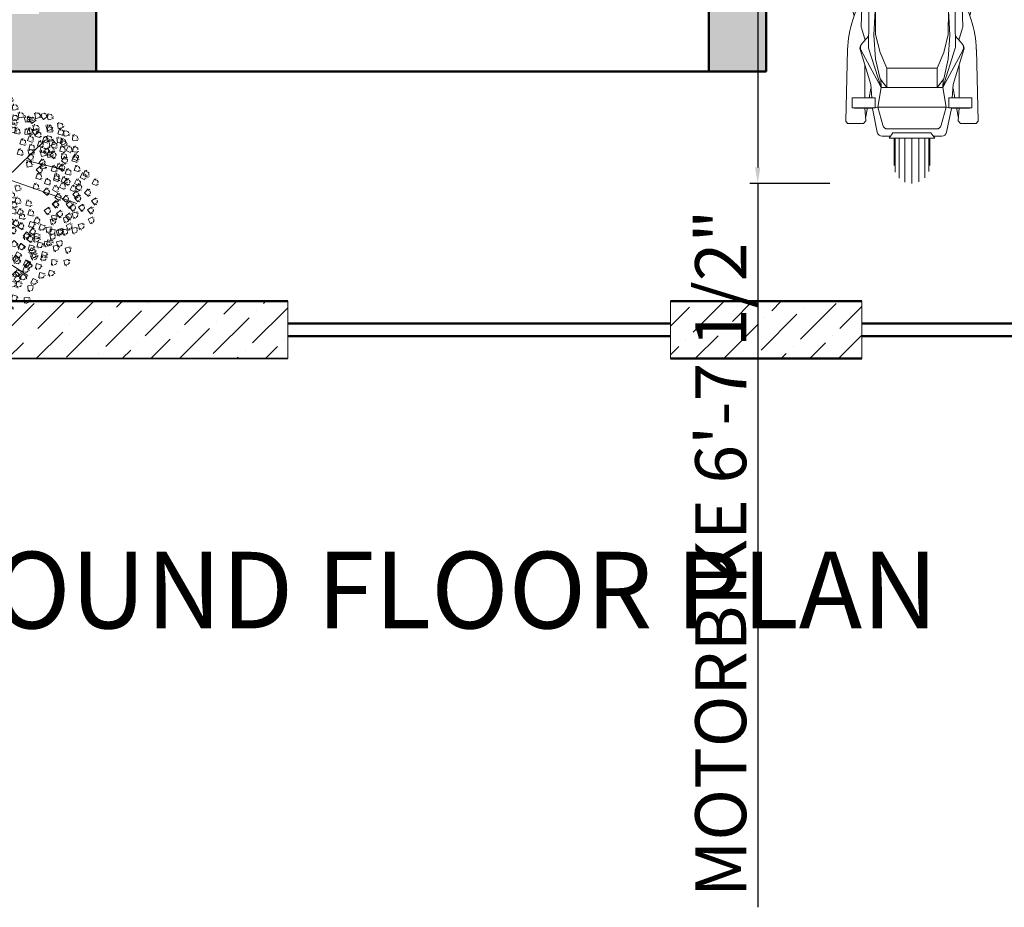
# Model space of a CAD drawing. Units: inches. Extents: x 3354 to 4308, y 1668 to 2317.
# Tile 2 of 11: x 3534 to 3689, y 1668 to 1807. Entities that reach past the tile are written whole.
import ezdxf

# ---------------------------------------------------------------- set-up
doc = ezdxf.new("R2010")
doc.units = ezdxf.units.IN
for name, color, linetype, lineweight in [('A-ANNO-DIMS', 2, 'Continuous', 18), ('A-ANNO-TEXT', 7, 'Continuous', 18), ('A-EQPM', 9, 'Continuous', 18), ('A-GLAZ', 4, 'Continuous', 18), ('A-WALL', 7, 'Continuous', 50), ('A-WALL-PATT', 8, 'Continuous', 13), ('C-PROP', 1, 'Continuous', 35), ('L-PLNT', 84, 'Continuous', 13)]:
    doc.layers.add(name, color=color, linetype=linetype, lineweight=lineweight)
doc.styles.get("Standard").update_dxf_attribs({"font": 'arial.ttf'})
doc.dimstyles.new('ISO-25', dxfattribs={"dimtxt": 8, "dimasz": 2.5, "dimexe": 1.25, "dimexo": 0.625, "dimtad": 1, "dimdec": 1, "dimlunit": 3, "dimtxsty": 'Standard', "dimcen": 2.5, "dimadec": 0, "dimazin": 0, "dimtfac": 1, "dimtdec": 1, "dimtmove": 0, "dimatfit": 3, "dimfxl": 1, "dimarcsym": 0})

# ---------------------------------------------------------------- blocks, each defined once
blk = doc.blocks.new('1 bike')
for p, q in [((-12.29, 42.13), (-12.29, 35.26)), ((-11.19, 35.26), (-11.19, 42.36)), ((-10.09, 42.17), (-10.09, 35.26)), ((-13.81, 35.26), (-13.81, 40.5)), ((-13.2, 41.5), (-13.2, 35.26)), ((-9.19, 41.55), (-9.19, 35.26)), ((-8.57, 35.26), (-8.57, 40.59)), ((-14.01, 39.55), (-14.01, 35.26)), ((-8.38, 39.55), (-8.38, 35.26)), ((-17.37, 30.6), (-16.62, 34.32)), ((-14.57, 34.95), (-15.85, 34.95)), ((-14.78, 35.24), (-14.17, 34.43)), ((-14.78, 35.24), (-7.6, 35.24)), ((-8.21, 34.43), (-14.17, 34.43)), ((-7.6, 35.24), (-8.21, 34.43)), ((-7.81, 34.95), (-6.53, 34.95)), ((-5.01, 30.6), (-5.76, 34.32)), ((-21.27, 32.95), (-21.54, 32.62)), ((-21.54, 32.62), (-21.28, 21.37)), ((-18.78, 32.95), (-21.27, 32.95)), ((-18.78, 32.95), (-18.43, 32.54)), ((-18.43, 32.54), (-18.57, 30.5)), ((-16.53, 30.42), (-15.78, 33.23)), ((-7.36, 33.82), (-15.02, 33.82)), ((-5.85, 30.42), (-6.6, 33.23)), ((-3.61, 32.95), (-3.95, 32.54)), ((-3.95, 32.54), (-3.81, 30.5)), ((-3.61, 32.95), (-1.11, 32.95)), ((-1.11, 32.95), (-0.84, 32.62)), ((-0.84, 32.62), (-1.1, 21.37)), ((-18.18, 30.5), (-18.46, 32.12)), ((-4.2, 30.5), (-3.92, 32.12)), ((-20.57, 28.93), (-20.57, 30.49)), ((-20.57, 30.49), (-16.95, 30.49)), ((-20.22, 30.58), (-17.31, 30.58)), ((-17.37, 30.5), (-17.37, 30.6)), ((-16.53, 30.42), (-17.37, 30.55)), ((-17.37, 30.55), (-17.37, 30.5)), ((-16.95, 30.49), (-16.95, 28.93)), ((-16.04, 27.32), (-16.53, 30.42)), ((-5.85, 30.42), (-16.5, 30.42)), ((-6.34, 27.32), (-5.85, 30.42)), ((-5.85, 30.42), (-5.01, 30.55)), ((-5.43, 30.49), (-5.43, 28.93)), ((-1.81, 30.49), (-5.43, 30.49)), ((-2.16, 30.58), (-5.08, 30.58)), ((-5.01, 30.5), (-5.01, 30.6)), ((-5.01, 30.55), (-5.01, 30.5)), ((-1.81, 28.93), (-1.81, 30.49)), ((-16.95, 28.93), (-20.57, 28.93)), ((-18.58, 28.93), (-18.58, 23.76)), ((-17.89, 28.92), (-17.63, 27.46)), ((-17.5, 28.92), (-17.66, 26.86)), ((-5.43, 28.93), (-1.81, 28.93)), ((-4.88, 28.92), (-4.72, 26.86)), ((-4.49, 28.92), (-4.75, 27.46)), ((-3.8, 28.93), (-3.8, 23.76)), ((-19.32, 21.36), (-17.66, 26.86)), ((-19.19, 21.42), (-16.04, 27.32)), ((-16.04, 27.32), (-17.98, 21.16)), ((-15.14, 27.32), (-16.17, 25.96)), ((-16.04, 27.32), (-16.08, 26.1)), ((-16.01, 27.32), (-6.34, 27.32)), ((-15.14, 24.28), (-15.14, 27.32)), ((-7.24, 27.32), (-6.21, 25.96)), ((-7.24, 24.28), (-7.24, 27.32)), ((-6.34, 27.32), (-6.31, 26.1)), ((-6.34, 27.32), (-4.4, 21.16)), ((-3.2, 21.42), (-6.34, 27.32)), ((-3.07, 21.36), (-4.72, 26.86)), ((-16.17, 25.96), (-16.89, 22.88)), ((-6.21, 25.96), (-5.5, 22.88)), ((-16.17, 21.85), (-15.14, 24.28)), ((-7.24, 24.28), (-15.11, 24.28)), ((-6.21, 21.85), (-7.24, 24.28)), ((-16.89, 22.88), (-17.14, 19.13)), ((-16.89, 19.03), (-16.17, 21.85)), ((-5.5, 19.03), (-6.21, 21.85)), ((-5.5, 22.88), (-5.24, 19.13)), ((-19.09, 20.53), (-18, 19.28)), ((-17.84, 6.18), (-18.02, 20.91)), ((-4.54, 6.18), (-4.37, 20.91)), ((-3.3, 20.53), (-4.39, 19.28)), ((-19.11, 17.99), (-18.54, 19.9)), ((-17.14, 19.13), (-16.46, 6.25)), ((-16.92, 15.02), (-16.89, 19.03)), ((-5.24, 19.13), (-5.92, 6.25)), ((-5.46, 15.02), (-5.5, 19.03)), ((-3.27, 17.99), (-3.84, 19.9)), ((-18.71, 5.16), (-19.15, 17.74)), ((-3.67, 5.16), (-3.24, 17.74)), ((-18.96, 12.28), (-20.45, 16.7)), ((-3.42, 12.28), (-1.93, 16.7)), ((-15.04, 6), (-16.92, 15.02)), ((-7.34, 6), (-5.46, 15.02)), ((-15.04, 6), (-16.46, 6.25)), ((-15.04, 6), (-16.46, 6.25)), ((-7.34, 6), (-5.92, 6.25)), ((-7.34, 6), (-5.92, 6.25)), ((-15.27, -8.98), (-15.04, 6)), ((-15.01, 6), (-7.34, 6)), ((-15.01, 6), (-7.34, 6)), ((-7.11, -8.98), (-7.34, 6)), ((-18.09, 2.47), (-18.58, 4.26)), ((-17.19, 4.06), (-16.68, 3.28)), ((-5.19, 4.06), (-5.71, 3.28)), ((-4.3, 2.47), (-3.81, 4.26)), ((-17.95, -6.66), (-17.95, 1.43)), ((-4.43, -6.66), (-4.43, 1.43)), ((-11.77, -3.74), (-12.84, -4.75)), ((-11.77, -3.74), (-10.61, -3.74)), ((-10.61, -3.74), (-9.54, -4.75)), ((-12.84, -4.75), (-12.84, -5.75)), ((-12.84, -5.75), (-11.77, -6.72)), ((-9.54, -5.75), (-10.61, -6.72)), ((-9.54, -4.75), (-9.54, -5.75)), ((-10.61, -6.72), (-11.77, -6.72)), ((-16.42, -11.25), (-17.67, -8.11)), ((-15.27, -8.98), (-16.42, -11.15)), ((-14.73, -11.31), (-15.27, -8.98)), ((-7.11, -8.98), (-15.24, -8.98)), ((-7.65, -11.31), (-7.11, -8.98)), ((-7.11, -8.98), (-5.96, -11.15)), ((-5.96, -11.25), (-4.71, -8.11)), ((-18.7, -12.25), (-19.45, -12.92)), ((-15.4, -15.97), (-18.7, -12.25)), ((-16.42, -11.15), (-16.42, -14.82)), ((-6.99, -15.97), (-3.68, -12.25)), ((-5.96, -11.15), (-5.96, -14.82)), ((-3.68, -12.25), (-2.93, -12.92)), ((-19.45, -12.92), (-16.84, -15.84)), ((-18.44, -12.54), (-19.19, -13.22)), ((-15.69, -15.57), (-14.92, -13.66)), ((-6.69, -15.57), (-7.46, -13.66)), ((-2.93, -12.92), (-5.54, -15.84)), ((-3.94, -12.54), (-3.19, -13.22)), ((-16.55, -15.97), (-15.4, -15.97)), ((-16.51, -15.99), (-15.16, -17.42)), ((-15.17, -16.45), (-15.61, -15.99)), ((-13.97, -16), (-13.29, -15.62)), ((-13.97, -16.52), (-13.97, -16)), ((-13.29, -16.91), (-13.97, -16.52)), ((-13.29, -16.1), (-13.75, -16.04)), ((-13.75, -16.36), (-13.29, -16.26)), ((-13.39, -15.74), (-13.1, -15.97)), ((-13.1, -16.42), (-13.39, -16.62)), ((-12.29, -15.62), (-13.29, -15.62)), ((-12.29, -16.91), (-13.29, -16.91)), ((-12.78, -15.91), (-12.78, -15.65)), ((-12.78, -16.49), (-12.78, -16.72)), ((-12.19, -15.74), (-12.45, -15.97)), ((-12.45, -16.42), (-12.19, -16.62)), ((-12.29, -15.62), (-11.58, -16)), ((-12.29, -16.91), (-11.58, -16.52)), ((-11.81, -16.04), (-12.26, -16.1)), ((-12.26, -16.26), (-11.81, -16.36)), ((-11.58, -16.52), (-11.58, -16)), ((-10.09, -15.62), (-10.8, -16)), ((-10.8, -16.52), (-10.8, -16)), ((-10.09, -16.91), (-10.8, -16.52)), ((-10.58, -16.04), (-10.12, -16.1)), ((-10.12, -16.26), (-10.58, -16.36)), ((-10.19, -15.74), (-9.93, -15.97)), ((-9.93, -16.42), (-10.19, -16.62)), ((-10.09, -15.62), (-9.09, -15.62)), ((-10.09, -16.91), (-9.09, -16.91)), ((-9.61, -15.91), (-9.61, -15.65)), ((-9.61, -16.49), (-9.61, -16.72)), ((-8.99, -15.74), (-9.28, -15.97)), ((-9.28, -16.42), (-8.99, -16.62)), ((-8.41, -16), (-9.09, -15.62)), ((-9.09, -16.1), (-8.64, -16.04)), ((-8.64, -16.36), (-9.09, -16.26)), ((-9.09, -16.91), (-8.41, -16.52)), ((-8.41, -16.52), (-8.41, -16)), ((-5.87, -15.99), (-7.22, -17.42)), ((-7.21, -16.45), (-6.77, -15.99)), ((-5.83, -15.97), (-6.99, -15.97)), ((-13.74, -17.07), (-8.65, -17.07)), ((-8.65, -18.04), (-13.73, -18.04)), ((-18.47, -24.58), (-18.47, -23.15)), ((-18.47, -23.15), (-16.35, -23.15)), ((-15.14, -24.58), (-18.47, -24.58)), ((-15.49, -24.67), (-18.15, -24.67)), ((-7.24, -24.58), (-3.91, -24.58)), ((-6.89, -24.67), (-4.24, -24.67)), ((-3.91, -23.15), (-6.03, -23.15)), ((-3.91, -24.58), (-3.91, -23.15)), ((-14.79, -24.85), (-14.79, -28.11)), ((-14.34, -25.16), (-14.62, -26.07)), ((-14.62, -26.07), (-14.62, -27.65)), ((-8.04, -25.18), (-7.76, -26.07)), ((-7.76, -26.07), (-7.76, -27.65)), ((-7.56, -24.85), (-7.56, -28.11)), ((-7.76, -27.65), (-14.62, -27.65)), ((-14.01, -30.38), (-14.01, -34.12)), ((-13.81, -35.22), (-13.81, -30.6)), ((-8.57, -35.22), (-8.57, -30.64)), ((-8.38, -30.42), (-8.38, -34.12)), ((-13.2, -31.13), (-13.2, -36.13)), ((-12.29, -36.74), (-12.29, -31.57)), ((-11.19, -31.75), (-11.19, -36.94)), ((-10.09, -36.74), (-10.09, -31.58)), ((-9.19, -31.15), (-9.19, -36.13))]:
    blk.add_line(p, q)
for centre, radius, start, end in [((-15.85, 34.16), 0.787, 90, 168.6493), ((-6.53, 34.16), 0.787, 11.3507, 90), ((-15.02, 33.03), 0.787, 90, 165.0682), ((-7.36, 33.03), 0.787, 14.9318, 90), ((-5.53, 21.74), 15.75, 181.3575, 198.6942), ((-18.56, 21.13), 0.787, 163.2719, 220.9137), ((-18.49, 21.05), 0.787, 151.9424, 220.9137), ((-17.23, 20.92), 0.787, 162.5452, 180.6944), ((-5.15, 20.92), 0.787, 359.3056, 17.4548), ((-3.89, 21.05), 0.787, 319.0863, 28.0576), ((-3.82, 21.13), 0.787, 319.0863, 16.7281), ((-16.85, 21.74), 15.75, 341.3058, 358.6425), ((-18.36, 17.77), 0.787, 163.359, 181.9702), ((-4.02, 17.77), 0.787, 358.0298, 16.641), ((39.63, 0), 62.01, 164.9421, 198.7675), ((-62.01, 0), 62.01, 341.2325, 15.0579), ((-13.9, 6.23), 3.94, 180.6944, 213.3274), ((43.19, 0.53), 59.93, 174.5142, 190.1132), ((-65.57, 0.53), 59.93, 349.8868, 5.4858), ((-8.48, 6.23), 3.94, 326.6726, 359.3056), ((-14.78, 5.3), 3.94, 181.9702, 195.2875), ((-7.6, 5.3), 3.94, 344.7125, 358.0298), ((-21.88, 1.43), 3.94, 0, 15.2875), ((-0.5, 1.43), 3.94, 164.7125, 180), ((-14.01, -6.66), 3.94, 180, 201.6868), ((-8.37, -6.66), 3.94, 338.3132, 0), ((-18.57, -12.19), 3.94, 338.094, 12.9179), ((-3.81, -12.19), 3.94, 167.0821, 201.906), ((-9.61, -9.24), 11.99, 197.8857, 221.2009), ((-12.77, -9.24), 11.99, 318.7991, 342.1143), ((-16.55, -15.58), 0.394, 221.8676, 270), ((-13.74, -15.1), 1.97, 223.2382, 270), ((-8.65, -15.1), 1.97, 270, 316.7618), ((-5.83, -15.58), 0.394, 270, 318.1324), ((-11.17, -8.43), 11.44, 229.5475, 310.4525), ((-13.73, -16.07), 1.97, 223.2382, 270), ((-8.65, -16.07), 1.97, 270, 316.7618), ((-11.17, -12.72), 10.69, 222.5562, 317.4438), ((-11.17, -20.07), 6, 196.0578, 343.9425), ((-11.17, -28.13), 3.61, 179.6687, 0.3313), ((-11.17, -34.14), 2.8, 179.6687, 0.3313)]:
    blk.add_arc(centre, radius, start, end)
blk = doc.blocks.new('3DLF-C')
for points, invisible_edges in [([(-3.5, -3.54, -3.54), (3.5, -3.54, -3.54), (0, 0)], 1), ([(-3, -4.99, -5.57), (3, -4.99, -5.57), (2, -3.54, -3.54), (-2, -3.54, -3.54)], 5), ([(0, -5.72, -7.43), (1.5, -4.99, -5.57), (-1.5, -4.99, -5.57)], 2)]:
    blk.add_3dface(points, dxfattribs=dict(invisible_edges=invisible_edges))
blk = doc.blocks.new('3DLFS-C')
for p in [(-0.5, 0, 16.75), (6.5, -6.75, 12), (-1.75, -11.41, 4.75), (-3, -20.04, -3.75), (5.75, -22.5)]:
    blk.add_blockref('3DLF-C', p)
for p, rotation in [((-21.75, -8.25, -0.46), 330.9453959009228), ((-8, -6.5, 10.5), 338.5232090204596), ((19.25, -4.75, 8.5), 25.76932762433872), ((-17.5, -13.5, 6.5), 339.0442232693679), ((12.25, -15, 3.25), 11.12918928961118), ((28, -11.58, 2.5), 29.93151184050779), ((-11.25, -21.75), 349.3803447238449), ((21.5, -20.96, 1), 29.93151184050779)]:
    blk.add_blockref('3DLF-C', p, dxfattribs=dict(rotation=rotation))
blk = doc.blocks.new('3DTREE1')
at = {"extrusion": (0, -1, -2e-16)}
for p, q in [((-39.3, 39, 219.3), (-16.2, 155, 282)), ((-71.7, 67.2, 244.1), (-65.7, 127.7, 299.9)), ((-39.3, 39, 216.3), (-108, 91.9, 268.4)), ((67, 1.4, 161.3), (144.2, 5.7, 213.8))]:
    blk.add_line(p, q, dxfattribs=at)
for p, q in [((63.6, 1.4, 162.1), (106.6, 94.5, 218.9)), ((-101.1, -15.6, 180.9), (-136.1, 16, 193.3)), ((64.8, 1.4, 162.1), (123.7, -61.7, 218.9)), ((-102, -16.5, 182.6), (-131.4, -38.6, 218.5)), ((-48, -36.8, 144.2), (-101.1, -15.6, 180.9)), ((123.7, -61.7, 218.9), (147.2, -24.6, 239.4)), ((-125, -111.6, 235.9), (-53.4, -42.5, 146.8)), ((-46.7, -36.8, 144.2), (-50.1, -109.9, 182.6)), ((123.7, -61.7, 218.9), (135.2, -99.2, 233.4))]:
    blk.add_line(p, q)
at = {"extrusion": (1, 0, 0)}
blk.add_line((-21.5, -34.8, 149.8), (-37, -26.3, 257.7), dxfattribs=at)
blk.add_lwpolyline([(13.2, 14.7, -0.117832), (14.5, 13, -0.109862), (14.9, 10.8, -0.036437), (14.7, 8.3, -0.034184), (14.1, 5.7, -0.070317), (13.2, 3.9, 0.121404), (12.8, 2.7, 0.105675), (12.9, 2, 0.10563), (13.2, 1.4, 0.11787), (14.1, 0.8, 0.050289), (16.6, 0.2, 0.018663), (18.9, -0.1, 0.01497), (21.7, -0.3, 0.087147), (23.7, 0, -0.118281), (25.2, 0.2, -0.325615), (26.3, -1, -0.326103), (25.6, -2.4, -0.032273), (24.2, -3, 0.027106), (22.6, -3.7, 0.002318), (19.2, -5.3, 0.008478), (18.3, -5.8, 0.036344), (17.3, -6.4, -0.022039), (15.8, -7.5, -0.092744), (13.2, -8.5, 0.069203), (9.8, -9.6, 0.147866), (7.6, -11.8, -0.172152), (5.5, -13.5, -0.132721), (3, -13.7, 0.108842), (0, -13.9, 0.053805), (-2.2, -14.8, -0.040641), (-5.1, -16, -0.081395), (-11.5, -17.1, -0.221332), (-13.7, -16, -0.079922), (-14.4, -14.9, -0.108313), (-14.5, -13.9, -0.048517), (-14.4, -12.8, -0.02389), (-13.7, -10.5, -0.137674), (-11.4, -7.3, 0.264867), (-10.7, -5.4, 0.017693), (-10.9, -4.2, 0.00755), (-11.5, -1.5, 0.004346), (-12.4, 1.8, 0.010497), (-12.8, 3.2, 0.070056), (-13.5, 4.6, 0.023562), (-16.2, 8.3, 0.090241), (-18.7, 10.4, -0.118501), (-20.5, 12.1, -0.08154), (-20.9, 13.1, -0.126697), (-20.9, 13.8, -0.215241), (-20.5, 14.4, -0.116434), (-19.2, 14.7, -0.22855), (-18, 14.1, 0.214017), (-16.7, 13.4, 0.07524), (-15.4, 13.5, 0.190759), (-15, 13.8, 0.274563), (-14.9, 14.4, -0.2385), (-15, 15.1, -0.087445), (-14.6, 15.7, -0.110244), (-14.1, 16, -0.136741), (-13.4, 16, -0.06456), (-12, 15.5, -0.144236), (-10.5, 14.2, 0.201708), (-9.4, 13.4, 0.026586), (-7.5, 13.1, -0.015616), (-4.3, 12.5, -0.012911), (-1, 11.8, 0.016293), (1.7, 11.3, 0.100723), (3.9, 11.3, 0.063874), (7.2, 12.5, 0.158892), (8.5, 13.9, -0.171356), (9.8, 15.1, -0.140353), (11.6, 15.4, -0.14068)], format="xyb", close=True)
at = {"elevation": 87.9}
for points in [[(0.4, 3.6), (-1.1, 3.4), (-2.6, 2.5), (-3.4, 1.7), (-4.1, 0.4), (-4.3, -1.1)], [(0.4, 3.6), (1.9, 3.4), (3.4, 2.5), (4.2, 1.7), (4.9, 0.4), (5.1, -1.1)], [(0.4, -5.8), (-1.1, -5.6), (-2.6, -4.7), (-3.4, -3.9), (-4.1, -2.6), (-4.3, -1.1)], [(0.4, -5.8), (1.9, -5.6), (3.4, -4.7), (4.2, -3.9), (4.9, -2.6), (5.1, -1.1)]]:
    blk.add_lwpolyline(points, dxfattribs=at)
for centre, radius in [((0.4, -1.1), 6.83), ((0.4, -1.1, 87.9), 4.69), ((0.8, -1.1, 86.6), 3.41)]:
    blk.add_circle(centre, radius)
at = {"extrusion": (0.668965, 0, 0.743294)}
blk.add_circle((1.6, 61.5, 163.4), 2.56, dxfattribs=at)
at = {"xscale": 1.706666666666666, "yscale": 1.706666666666666, "zscale": 1.706666666666666}
for name, p, rotation in [('3DLFS-C', (-13.6, 138.7, 209.1), 180), ('3DLFS-C', (-50.3, 113, 288.1), 217.0355451173859), ('3DLFS-C', (68.8, 96.4, 191.6), 127.0355451173859), ('3DLFS-C', (-90.3, 99.3, 187.4), 241.10908773184), ('3DLFS-C', (21.9, 87, 153.2), 127.0355451173859), ('3DLFS-C', (41.5, 81.2, 271.8), 127.0355451173859), ('3DLFS-C', (-89, 85.2, 227), 217.0355451173859), ('3DLFS-C', (-30.5, 83, 187.3), 217.0355451173859), ('3DLFS-C', (1, 105.9, 248.4), 180), ('3DLFS-C', (-80.4, 50.7, 249.2), 217.0355451173859), ('3DLFS-C', (28.8, 51.1, 172), 217.0355451173859), ('3DLFS-C', (126.8, 45.3, 236), 116.7371100578058), ('3DLFS-C', (64.3, 39.8, 138.3), 90), ('3DLFS-C', (73.7, 39.8, 300.3), 90), ('3DLFS-C', (-108.7, 24.8, 134.8), 241.10908773184), ('3DLFS-C', (19.6, 23.1, 316.2), 217.0355451173859), ('3DLFS-C', (113.3, 18.1, 166.2), 105.1767250495332), ('3DLFS-C', (41.6, -10, 304.8), 127.0355451173859), ('3DLFS-C', (-101.5, -0.4, 274.2), 274.426310174705), ('3DLFS-C', (-141, -10.4, 198.6), 274.426310174705), ('3DLFS-C', (76.2, -35.1, 240.2), 105.1767250495332), ('3DLFS-C', (-154.1, -35.2, 230.9), 260.280514680602), ('3DLFS-C', (-36, -5.1, 325.5), 311.4618552920909), ('3DLFS-C', (-54.5, -35.2, 179.4), 274.426310174705), ('3DLFS-C', (-90, -43.3, 295.7), 311.4618552920909), ('3DLF-C', (-20.6, -4.1, 353.7), 319.1446237411043), ('3DLFS-C', (116.7, -67.8, 211.5), 68.14117993214732), ('3DLF-C', (14.1, -21.6, 363.3), 46.3875157474432), ('3DLFS-C', (-59.6, -89, 158.7), 294.8881552746311), ('3DLFS-C', (-17.8, -65, 244.3), 342.4928092333246), ('3DLFS-C', (-17.8, -80.2, 257.5), 342.4928092333246), ('3DLFS-C', (-25.2, -86.2, 179.4), 351.3217393776923), ('3DLFS-C', (48.4, -119.8, 204.2), 20.68147253157148), ('3DLFS-C', (62.7, -113.9, 272.2), 19.52835435071045), ('3DLFS-C', (38.6, -131.8, 232.1), 19.52835435071045)]:
    blk.add_blockref(name, p, dxfattribs=dict(at, rotation=rotation))
blk.add_blockref('3DLF-C', (3.3, -21.6, 352.8), dxfattribs=at)
mesh = blk.add_polymesh((2, 36), dxfattribs=dict(n_close=True))
for k, corner in enumerate([(-1.5, 0.6, 84.1), (-1, 1, 84.1), (-0.5, 1.4, 84.1), (0.1, 1.6, 84.1), (0.6, 1.7, 84.1), (1.2, 1.7, 84.1), (1.8, 1.6, 84.1), (2.4, 1.4, 84.1), (2.9, 1.1, 84.1), (3.4, 0.8, 84.1), (3.8, 0.3, 84.1), (4.1, -0.2, 84.1), (4.3, -0.7, 84.1), (4.4, -1.3, 84.1), (4.4, -1.9, 84.1), (4.3, -2.5, 84.1), (4.2, -3.1, 84.1), (3.9, -3.6, 84.1), (3.5, -4.1, 84.1), (3.1, -4.4, 84.1), (2.5, -4.8, 84.1), (2, -5, 84.1), (1.4, -5.1, 84.1), (0.8, -5.1, 84.1), (0.2, -5, 84.1), (-0.3, -4.8, 84.1), (-0.9, -4.5, 84.1), (-1.3, -4.2, 84.1), (-1.7, -3.7, 84.1), (-2, -3.2, 84.1), (-2.2, -2.7, 84.1), (-2.4, -2.1, 84.1), (-2.4, -1.5, 84.1), (-2.3, -0.9, 84.1), (-2.1, -0.3, 84.1), (-1.8, 0.2, 84.1), (-38.4, 38.9, 216.7), (-38.2, 38.6, 217), (-38, 38.3, 217.3), (-37.9, 38, 217.6), (-37.9, 37.6, 217.8), (-38, 37.2, 218.1), (-38.1, 36.8, 218.2), (-38.3, 36.4, 218.4), (-38.5, 36, 218.4), (-38.8, 35.7, 218.5), (-39.1, 35.4, 218.4), (-39.5, 35.1, 218.4), (-39.8, 34.9, 218.2), (-40.2, 34.8, 218.1), (-40.6, 34.7, 217.8), (-41, 34.7, 217.6), (-41.3, 34.8, 217.3), (-41.7, 34.9, 217), (-41.9, 35.1, 216.7), (-42.1, 35.4, 216.4), (-42.3, 35.7, 216.2), (-42.4, 36.1, 215.9), (-42.4, 36.4, 215.6), (-42.4, 36.8, 215.4), (-42.2, 37.2, 215.3), (-42.1, 37.6, 215.1), (-41.8, 38, 215.1), (-41.5, 38.3, 215), (-41.2, 38.6, 215.1), (-40.9, 38.9, 215.1), (-40.5, 39.1, 215.3), (-40.1, 39.2, 215.4), (-39.7, 39.3, 215.6), (-39.3, 39.3, 215.9), (-39, 39.2, 216.2), (-38.7, 39.1, 216.4)]):
    mesh.set_mesh_vertex(divmod(k, 36), corner)
mesh = blk.add_polymesh((2, 36), dxfattribs=dict(n_close=True))
for k, corner in enumerate([(-1.5, 0.6, 84.1), (-1, 1, 84.1), (-0.5, 1.4, 84.1), (0.1, 1.6, 84.1), (0.6, 1.7, 84.1), (1.2, 1.7, 84.1), (1.8, 1.6, 84.1), (2.4, 1.4, 84.1), (2.9, 1.1, 84.1), (3.4, 0.8, 84.1), (3.8, 0.3, 84.1), (4.1, -0.2, 84.1), (4.3, -0.7, 84.1), (4.4, -1.3, 84.1), (4.4, -1.9, 84.1), (4.3, -2.5, 84.1), (4.2, -3.1, 84.1), (3.9, -3.6, 84.1), (3.5, -4.1, 84.1), (3.1, -4.4, 84.1), (2.5, -4.8, 84.1), (2, -5, 84.1), (1.4, -5.1, 84.1), (0.8, -5.1, 84.1), (0.2, -5, 84.1), (-0.3, -4.8, 84.1), (-0.9, -4.5, 84.1), (-1.3, -4.2, 84.1), (-1.7, -3.7, 84.1), (-2, -3.2, 84.1), (-2.2, -2.7, 84.1), (-2.4, -2.1, 84.1), (-2.4, -1.5, 84.1), (-2.3, -0.9, 84.1), (-2.1, -0.3, 84.1), (-1.8, 0.2, 84.1), (-38.4, 38.9, 216.7), (-38.2, 38.6, 217), (-38, 38.3, 217.3), (-37.9, 38, 217.6), (-37.9, 37.6, 217.8), (-38, 37.2, 218.1), (-38.1, 36.8, 218.2), (-38.3, 36.4, 218.4), (-38.5, 36, 218.4), (-38.8, 35.7, 218.5), (-39.1, 35.4, 218.4), (-39.5, 35.1, 218.4), (-39.8, 34.9, 218.2), (-40.2, 34.8, 218.1), (-40.6, 34.7, 217.8), (-41, 34.7, 217.6), (-41.3, 34.8, 217.3), (-41.7, 34.9, 217), (-41.9, 35.1, 216.7), (-42.1, 35.4, 216.4), (-42.3, 35.7, 216.2), (-42.4, 36.1, 215.9), (-42.4, 36.4, 215.6), (-42.4, 36.8, 215.4), (-42.2, 37.2, 215.3), (-42.1, 37.6, 215.1), (-41.8, 38, 215.1), (-41.5, 38.3, 215), (-41.2, 38.6, 215.1), (-40.9, 38.9, 215.1), (-40.5, 39.1, 215.3), (-40.1, 39.2, 215.4), (-39.7, 39.3, 215.6), (-39.3, 39.3, 215.9), (-39, 39.2, 216.2), (-38.7, 39.1, 216.4)]):
    mesh.set_mesh_vertex(divmod(k, 36), corner)
mesh = blk.add_polymesh((2, 36), dxfattribs=dict(n_close=True))
for k, corner in enumerate([(7.2, -1.1), (7.1, 0.1), (6.8, 1.2), (6.3, 2.3), (5.6, 3.3), (4.8, 4.1), (3.8, 4.8), (2.7, 5.3), (1.6, 5.6), (0.4, 5.7), (-0.8, 5.6), (-1.9, 5.3), (-3, 4.8), (-4, 4.1), (-4.8, 3.3), (-5.5, 2.3), (-6, 1.2), (-6.3, 0.1), (-6.4, -1.1), (-6.3, -2.3), (-6, -3.4), (-5.5, -4.5), (-4.8, -5.5), (-4, -6.3), (-3, -7), (-1.9, -7.5), (-0.8, -7.8), (0.4, -7.9), (1.6, -7.8), (2.7, -7.5), (3.8, -7), (4.8, -6.3), (5.6, -5.5), (6.3, -4.5), (6.8, -3.4), (7.1, -2.3), (9.4, 14.9, -23.9), (6.4, 12.2, -23.9), (2.5, 11.2, -23.9), (-1.5, 11.9, -23.9), (-5.5, 12.8, -23.9), (-9.6, 13.4, -23.9), (-12.8, 15.8, -23.9), (-15, 13.7, -23.9), (-18.7, 14.6, -23.9), (-20.6, 12.4, -23.9), (-17.6, 9.7, -23.9), (-14.9, 6.6, -23.9), (-12.8, 3.1, -23.9), (-11.7, -0.8, -23.9), (-10.8, -4.8, -23.9), (-12.4, -8.3, -23.9), (-14.1, -11.9, -23.9), (-13.9, -15.8, -23.9), (-10.2, -17, -23.9), (-6.2, -16.4, -23.9), (-2.4, -14.9, -23.9), (1.5, -13.7, -23.9), (5.6, -13.5, -23.9), (8.4, -10.6, -23.9), (12, -8.8, -23.9), (15.9, -7.5, -23.9), (19.3, -5.3, -23.9), (23, -3.5, -23.9), (26.3, -1.4, -23.9), (23.2, -0.1, -23.9), (19.2, -0.1, -23.9), (15.1, 0.5, -23.9), (12.9, 3.3, -23.9), (14.4, 7, -23.9), (14.9, 11.1, -23.9), (13.2, 14.7, -23.9)]):
    mesh.set_mesh_vertex(divmod(k, 36), corner)
mesh = blk.add_polymesh((2, 36), dxfattribs=dict(n_close=True))
for k, corner in enumerate([(-1.5, -2.8, 84.1), (-1.9, -2.3, 84.1), (-2.1, -1.8, 84.1), (-2.3, -1.2, 84.1), (-2.4, -0.7, 84.1), (-2.3, -0.1, 84.1), (-2.2, 0.5, 84.1), (-2, 1.1, 84.1), (-1.6, 1.6, 84.1), (-1.2, 2, 84.1), (-0.8, 2.4, 84.1), (-0.2, 2.6, 84.1), (0.3, 2.8, 84.1), (0.9, 2.9, 84.1), (1.5, 2.8, 84.1), (2.1, 2.7, 84.1), (2.6, 2.5, 84.1), (3.1, 2.1, 84.1), (3.6, 1.7, 84.1), (3.9, 1.3, 84.1), (4.2, 0.7, 84.1), (4.4, 0.2, 84.1), (4.5, -0.4, 84.1), (4.4, -1, 84.1), (4.3, -1.6, 84.1), (4.1, -2.1, 84.1), (3.7, -2.6, 84.1), (3.3, -3.1, 84.1), (2.8, -3.4, 84.1), (2.3, -3.7, 84.1), (1.7, -3.9, 84.1), (1.2, -4, 84.1), (0.6, -3.9, 84.1), (0, -3.8, 84.1), (-0.6, -3.6, 84.1), (-1.1, -3.2, 84.1), (-55.7, -36.2, 146.8), (-55.4, -36, 147.1), (-55.1, -35.9, 147.4), (-54.7, -35.8, 147.6), (-54.3, -35.8, 147.9), (-54, -35.9, 148.1), (-53.6, -36.1, 148.3), (-53.2, -36.3, 148.4), (-52.8, -36.5, 148.5), (-52.5, -36.9, 148.5), (-52.3, -37.2, 148.5), (-52, -37.6, 148.4), (-51.9, -38, 148.3), (-51.8, -38.4, 148.1), (-51.7, -38.8, 147.9), (-51.8, -39.1, 147.6), (-51.9, -39.5, 147.4), (-52, -39.8, 147.1), (-52.2, -40, 146.8), (-52.5, -40.2, 146.5), (-52.8, -40.3, 146.2), (-53.2, -40.4, 145.9), (-53.5, -40.4, 145.7), (-53.9, -40.3, 145.5), (-54.3, -40.2, 145.3), (-54.7, -40, 145.2), (-55, -39.7, 145.1), (-55.4, -39.4, 145.1), (-55.6, -39, 145.1), (-55.9, -38.7, 145.2), (-56, -38.3, 145.3), (-56.1, -37.9, 145.5), (-56.2, -37.5, 145.7), (-56.1, -37.1, 145.9), (-56, -36.8, 146.2), (-55.9, -36.5, 146.5)]):
    mesh.set_mesh_vertex(divmod(k, 36), corner)
mesh = blk.add_polymesh((2, 36), dxfattribs=dict(n_close=True))
for k, corner in enumerate([(-1.5, -2.8, 84.1), (-1.9, -2.3, 84.1), (-2.1, -1.8, 84.1), (-2.3, -1.2, 84.1), (-2.4, -0.7, 84.1), (-2.3, -0.1, 84.1), (-2.2, 0.5, 84.1), (-2, 1.1, 84.1), (-1.6, 1.6, 84.1), (-1.2, 2, 84.1), (-0.8, 2.4, 84.1), (-0.2, 2.6, 84.1), (0.3, 2.8, 84.1), (0.9, 2.9, 84.1), (1.5, 2.8, 84.1), (2.1, 2.7, 84.1), (2.6, 2.5, 84.1), (3.1, 2.1, 84.1), (3.6, 1.7, 84.1), (3.9, 1.3, 84.1), (4.2, 0.7, 84.1), (4.4, 0.2, 84.1), (4.5, -0.4, 84.1), (4.4, -1, 84.1), (4.3, -1.6, 84.1), (4.1, -2.1, 84.1), (3.7, -2.6, 84.1), (3.3, -3.1, 84.1), (2.8, -3.4, 84.1), (2.3, -3.7, 84.1), (1.7, -3.9, 84.1), (1.2, -4, 84.1), (0.6, -3.9, 84.1), (0, -3.8, 84.1), (-0.6, -3.6, 84.1), (-1.1, -3.2, 84.1), (-53.9, -39.6, 146.8), (-53.7, -39.4, 147.1), (-53.4, -39.3, 147.4), (-53, -39.3, 147.6), (-52.6, -39.3, 147.9), (-52.3, -39.3, 148.1), (-51.9, -39.5, 148.3), (-51.5, -39.7, 148.4), (-51.1, -40, 148.5), (-50.8, -40.3, 148.5), (-50.5, -40.6, 148.5), (-50.3, -41, 148.4), (-50.2, -41.4, 148.3), (-50.1, -41.8, 148.1), (-50, -42.2, 147.9), (-50, -42.6, 147.6), (-50.1, -42.9, 147.4), (-50.3, -43.2, 147.1), (-50.5, -43.4, 146.8), (-50.8, -43.6, 146.5), (-51.1, -43.8, 146.2), (-51.5, -43.8, 145.9), (-51.8, -43.8, 145.7), (-52.2, -43.7, 145.5), (-52.6, -43.6, 145.3), (-53, -43.4, 145.2), (-53.3, -43.1, 145.1), (-53.7, -42.8, 145.1), (-53.9, -42.5, 145.1), (-54.2, -42.1, 145.2), (-54.3, -41.7, 145.3), (-54.4, -41.3, 145.5), (-54.5, -40.9, 145.7), (-54.4, -40.5, 145.9), (-54.3, -40.2, 146.2), (-54.2, -39.9, 146.5)]):
    mesh.set_mesh_vertex(divmod(k, 36), corner)
mesh = blk.add_polymesh((2, 36), dxfattribs=dict(n_close=True))
for k, corner in enumerate([(7.2, -1.1), (7.1, 0.1), (6.8, 1.2), (6.3, 2.3), (5.6, 3.3), (4.8, 4.1), (3.8, 4.8), (2.7, 5.3), (1.6, 5.6), (0.4, 5.7), (-0.8, 5.6), (-1.9, 5.3), (-3, 4.8), (-4, 4.1), (-4.8, 3.3), (-5.5, 2.3), (-6, 1.2), (-6.3, 0.1), (-6.4, -1.1), (-6.3, -2.3), (-6, -3.4), (-5.5, -4.5), (-4.8, -5.5), (-4, -6.3), (-3, -7), (-1.9, -7.5), (-0.8, -7.8), (0.4, -7.9), (1.6, -7.8), (2.7, -7.5), (3.8, -7), (4.8, -6.3), (5.6, -5.5), (6.3, -4.5), (6.8, -3.4), (7.1, -2.3), (5.1, -1.1, 87.9), (5, -0.3, 87.9), (4.8, 0.5, 87.9), (4.5, 1.2, 87.9), (4, 1.9, 87.9), (3.4, 2.5, 87.9), (2.8, 3, 87.9), (2, 3.3, 87.9), (1.2, 3.5, 87.9), (0.4, 3.6, 87.9), (-0.4, 3.5, 87.9), (-1.2, 3.3, 87.9), (-1.9, 3, 87.9), (-2.6, 2.5, 87.9), (-3.2, 1.9, 87.9), (-3.7, 1.2, 87.9), (-4, 0.5, 87.9), (-4.2, -0.3, 87.9), (-4.3, -1.1, 87.9), (-4.2, -1.9, 87.9), (-4, -2.7, 87.9), (-3.7, -3.5, 87.9), (-3.2, -4.1, 87.9), (-2.6, -4.7, 87.9), (-1.9, -5.2, 87.9), (-1.2, -5.5, 87.9), (-0.4, -5.7, 87.9), (0.4, -5.8, 87.9), (1.2, -5.7, 87.9), (2, -5.5, 87.9), (2.8, -5.2, 87.9), (3.4, -4.7, 87.9), (4, -4.1, 87.9), (4.5, -3.5, 87.9), (4.8, -2.7, 87.9), (5, -1.9, 87.9)]):
    mesh.set_mesh_vertex(divmod(k, 36), corner)
mesh = blk.add_polymesh((2, 36), dxfattribs=dict(n_close=True))
for k, corner in enumerate([(4.2, -1.1, 86.6), (4.2, -0.5, 86.6), (4, 0.1, 86.6), (3.8, 0.6, 86.6), (3.4, 1.1, 86.6), (3, 1.5, 86.6), (2.5, 1.8, 86.6), (2, 2.1, 86.6), (1.4, 2.2, 86.6), (0.8, 2.3, 86.6), (0.2, 2.2, 86.6), (-0.3, 2.1, 86.6), (-0.9, 1.8, 86.6), (-1.4, 1.5, 86.6), (-1.8, 1.1, 86.6), (-2.1, 0.6, 86.6), (-2.4, 0.1, 86.6), (-2.5, -0.5, 86.6), (-2.6, -1.1, 86.6), (-2.5, -1.7, 86.6), (-2.4, -2.3, 86.6), (-2.1, -2.8, 86.6), (-1.8, -3.3, 86.6), (-1.4, -3.7, 86.6), (-0.9, -4.1, 86.6), (-0.3, -4.3, 86.6), (0.2, -4.5, 86.6), (0.8, -4.5, 86.6), (1.4, -4.5, 86.6), (2, -4.3, 86.6), (2.5, -4.1, 86.6), (3, -3.7, 86.6), (3.4, -3.3, 86.6), (3.8, -2.8, 86.6), (4, -2.3, 86.6), (4.2, -1.7, 86.6), (63.6, 4.2, 162.6), (63.3, 4.1, 162.9), (62.9, 4, 163.1), (62.6, 3.8, 163.4), (62.4, 3.6, 163.7), (62.1, 3.2, 163.9), (61.9, 2.9, 164), (61.8, 2.5, 164.2), (61.7, 2, 164.2), (61.7, 1.6, 164.3), (61.7, 1.2, 164.2), (61.8, 0.7, 164.2), (61.9, 0.3, 164), (62.1, 0, 163.9), (62.4, -0.4, 163.7), (62.6, -0.6, 163.4), (62.9, -0.8, 163.1), (63.3, -0.9, 162.9), (63.6, -1, 162.6), (63.9, -0.9, 162.3), (64.2, -0.8, 162), (64.5, -0.6, 161.7), (64.8, -0.4, 161.5), (65.1, 0, 161.2), (65.2, 0.3, 161.1), (65.4, 0.7, 160.9), (65.5, 1.2, 160.9), (65.5, 1.6, 160.8), (65.5, 2, 160.9), (65.4, 2.5, 160.9), (65.2, 2.9, 161.1), (65.1, 3.2, 161.2), (64.8, 3.6, 161.5), (64.5, 3.8, 161.7), (64.2, 4, 162), (63.9, 4.1, 162.3)]):
    mesh.set_mesh_vertex(divmod(k, 36), corner)
blk = doc.blocks.new('*D72')
at = {"layer": 'A-ANNO-DIMS', "color": 0, "lineweight": -2, "transparency": 16777216}
for p, q in [((3661.24, 1861.18), (3648.7, 1861.18)), ((3649.95, 1858.68), (3649.95, 1784.26)), ((3661.24, 1781.76), (3648.7, 1781.76)), ((3649.95, 1781.76), (3649.95, 1668.3))]:
    blk.add_line(p, q, dxfattribs=at)
at = {"layer": 'A-ANNO-DIMS', "color": 0, "transparency": 16777216}
for points in [[(3649.53, 1858.68), (3650.36, 1858.68), (3649.95, 1861.18)], [(3649.53, 1784.26), (3650.36, 1784.26), (3649.95, 1781.76)]]:
    blk.add_solid(points, dxfattribs=at)
at = {"layer": 'Defpoints', "color": 0, "transparency": 16777216}
for p in [(3661.86, 1861.18), (3649.95, 1781.76), (3661.86, 1781.76)]:
    blk.add_point(p, dxfattribs=at)
at = {"layer": 'A-ANNO-DIMS', "color": 0, "transparency": 16777216, "insert": (3645.18, 1723.78), "char_height": 8, "attachment_point": 5, "rotation": 90}
blk.add_mtext('MOTORBIKE 6\'-7 1/2"', dxfattribs=at)

msp = doc.modelspace()

# ---------------------------------------------------------------- hatches: boundary and pattern name
at = {"layer": 'A-WALL-PATT', "transparency": 33554687}
h = msp.add_hatch(color=256, dxfattribs=at)
h.dxf.hatch_style = 1
h.paths.add_polyline_path([(3546.28, 1829.3), (3552.28, 1829.3), (3552.28, 1838.3), (3546.28, 1838.3), (3546.28, 1910.3), (3582.28, 1910.3), (3582.28, 1919.3), (3546.28, 1919.3), (3546.28, 1961.3), (3534.28, 1961.3), (3534.28, 1955.3), (3537.28, 1955.3), (3537.28, 1808.3), (3516.28, 1808.3), (3516.28, 1799.3), (3546.28, 1799.3)])
h.paths.add_polyline_path([(3672.28, 1919.3), (3656.51, 1919.3), (3630.28, 1919.3), (3630.28, 1910.3), (3642.28, 1910.3), (3642.28, 1838.3), (3630.28, 1838.3), (3630.28, 1835.3), (3630.28, 1829.3), (3642.28, 1829.3), (3642.28, 1799.3), (3651.28, 1799.3), (3651.28, 1910.3), (3672.28, 1910.3)])
h.paths.add_polyline_path([(3744.28, 1959.8), (3735.28, 1959.8), (3735.28, 1923.23), (3735.28, 1919.3), (3714.28, 1919.3), (3714.28, 1910.3), (3744.28, 1910.3)])
h.paths.add_polyline_path([(3744.28, 2072.3), (3735.28, 2072.3), (3735.28, 2031.8), (3744.28, 2031.8)])
h.paths.add_polyline_path([(3744.28, 2150.3), (3735.28, 2150.3), (3735.28, 2108.3), (3744.28, 2108.3)])
h.paths.add_polyline_path([(3744.28, 2258.3), (3705.28, 2258.3), (3705.28, 2249.3), (3735.28, 2249.3), (3735.28, 2210.3), (3744.28, 2210.3)])
h.paths.add_polyline_path([(3633.28, 2258.3), (3583.78, 2258.3), (3583.78, 2249.3), (3588.24, 2249.3), (3597.28, 2249.3), (3597.28, 2165.3), (3594.28, 2165.3), (3594.28, 2159.3), (3597.28, 2159.3), (3597.28, 2117.3), (3594.28, 2117.3), (3594.28, 2111.3), (3603.28, 2111.3), (3603.28, 2249.3), (3633.28, 2249.3)])
h.paths.add_polyline_path([(3559.78, 2258.3), (3492.28, 2258.3), (3492.28, 2249.3), (3537.28, 2249.3), (3537.28, 2117.3), (3534.28, 2117.3), (3534.28, 2111.3), (3564.28, 2111.3), (3564.28, 2117.3), (3546.28, 2117.3), (3546.28, 2159.3), (3564.28, 2159.3), (3564.28, 2165.3), (3546.28, 2165.3), (3546.28, 2249.3), (3559.78, 2249.3)])
h.paths.add_polyline_path([(3450.28, 2258.3), (3396.28, 2258.3), (3396.28, 1799.3), (3474.28, 1799.3), (3474.28, 1808.3), (3405.28, 1808.3), (3405.28, 1955.3), (3498.28, 1955.3), (3498.28, 1961.3), (3405.28, 1961.3), (3405.28, 2111.3), (3498.28, 2111.3), (3498.28, 2117.3), (3405.28, 2117.3), (3405.28, 2249.3), (3450.28, 2249.3)])
h.paths.add_polyline_path([(3582.28, 1838.3), (3576.28, 1838.3), (3576.28, 1829.3), (3582.28, 1829.3)], flags=17)
h = msp.add_hatch(dxfattribs=at)
h.set_pattern_fill('ANSI36', color=256)
h.paths.add_polyline_path([(3576.28, 1763.3), (3405.28, 1763.3), (3405.28, 1799.3), (3396.28, 1799.3), (3396.28, 1754.3), (3576.28, 1754.3)])
h = msp.add_hatch(dxfattribs=at)
h.set_pattern_fill('ANSI36', color=256)
h.paths.add_polyline_path([(3666.28, 1763.3), (3636.28, 1763.3), (3636.28, 1754.3), (3666.28, 1754.3)])
h.paths.add_polyline_path([(3780.28, 1763.3), (3738.28, 1763.3), (3738.28, 1754.3), (3780.28, 1754.3)])

# ---------------------------------------------------------------- linework, layer by layer
at = {"layer": 'A-GLAZ'}
for p, q in [((3576.28, 1763.3), (3576.28, 1754.3)), ((3636.28, 1763.3), (3636.28, 1754.3)), ((3666.28, 1763.3), (3666.28, 1754.3))]:
    msp.add_line(p, q, dxfattribs=at)
at = {"layer": 'A-WALL'}
for p, q in [((3651.28, 1910.3), (3651.28, 1799.3)), ((3546.28, 1829.3), (3546.28, 1799.3)), ((3642.28, 1829.3), (3642.28, 1799.3)), ((3396.28, 1799.3), (3651.28, 1799.3)), ((3405.28, 1763.3), (3576.28, 1763.3)), ((3636.28, 1763.3), (3666.28, 1763.3)), ((3576.28, 1759.8), (3636.28, 1759.8)), ((3666.28, 1759.8), (3738.28, 1759.8)), ((3576.28, 1757.8), (3636.28, 1757.8)), ((3666.28, 1757.8), (3738.28, 1757.8))]:
    msp.add_line(p, q, dxfattribs=at)
msp.add_lwpolyline([(3636.28, 1754.3), (3666.28, 1754.3)], dxfattribs=at)
at = {"layer": 'C-PROP'}
msp.add_lwpolyline([(3738.28, 1754.3), (3780.28, 1754.3), (3780.28, 2294.3), (3396.28, 2294.3), (3396.28, 1754.3), (3576.28, 1754.3)], dxfattribs=at)

# ---------------------------------------------------------------- block references
at = {"layer": 'A-EQPM', "rotation": 180}
msp.add_blockref('1 bike', (3662.93, 1824.12), dxfattribs=at)
at = {"layer": 'L-PLNT', "xscale": 0.0998176642374887, "yscale": 0.0998176642374887, "zscale": 0.0998176642374887, "rotation": 261.8658016160191}
msp.add_blockref('3DTREE1', (3527.7, 1779.21, -18.18), dxfattribs=at)

# ---------------------------------------------------------------- texts
at = {"layer": 'A-ANNO-TEXT', "insert": (3508.44, 1724.02), "char_height": 12, "attachment_point": 1}
msp.add_mtext_dynamic_manual_height_columns('GROUND FLOOR PLAN', width=202.1172, gutter_width=12.5, heights=[0], dxfattribs=at)

# ---------------------------------------------------------------- dimensions: what is measured, and where the dimension line sits
at = {"layer": 'A-ANNO-DIMS'}
dim = msp.add_linear_dim(base=(3649.95, 1781.76), p1=(3661.86, 1861.18), p2=(3661.86, 1781.76), angle=270, text='MOTORBIKE <>', dimstyle='ISO-25', override={"dimdec": 1, "dimrnd": 0, "dimzin": 1, "dimlunit": 4, "dimfrac": 2}, dxfattribs=at)
dim.commit()
dim.dimension.update_dxf_attribs({"geometry": '*D72', "text_midpoint": (3645.18, 1723.78)})

doc.saveas('drawing.dxf')
